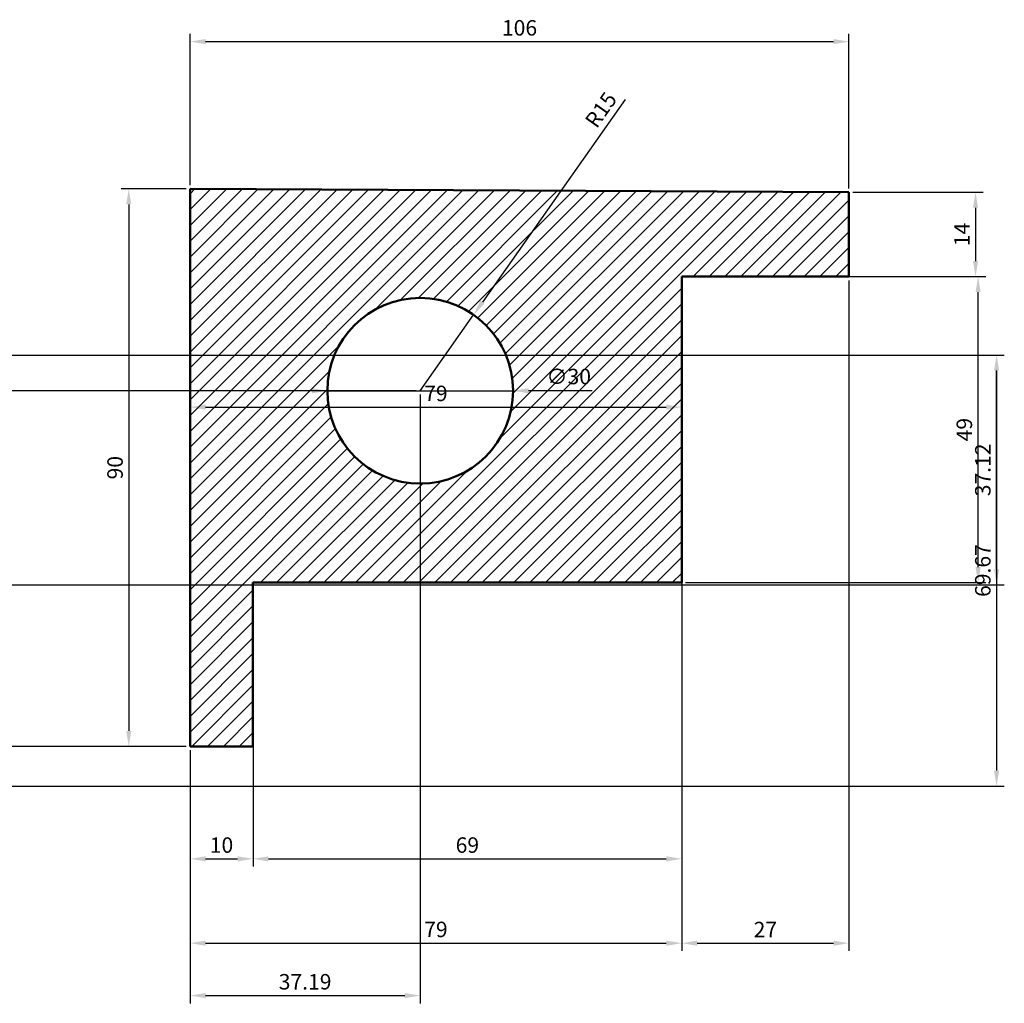
# Model space of a CAD drawing. Units: millimetres. Extents: x 1605 to 2079, y 1280 to 1879.
# Tile 6 of 7: x 1920 to 2079, y 1384 to 1543. Entities that reach past the tile are written whole.
import ezdxf

# ---------------------------------------------------------------- set-up
doc = ezdxf.new("R2010")
doc.units = ezdxf.units.MM
for name, color, linetype, lineweight in [('M-DIMS', 2, 'Continuous', 25), ('M-HATC', 8, 'Continuous', 18), ('M-OUTL', 7, 'Continuous', 50)]:
    doc.layers.add(name, color=color, linetype=linetype, lineweight=lineweight)
doc.styles.get("Standard").update_dxf_attribs({"font": 'arial.ttf'})
doc.dimstyles.new('ISO-25', dxfattribs={"dimtxt": 2.5, "dimasz": 2.5, "dimexe": 1.25, "dimexo": 0.625, "dimtad": 1, "dimdec": 0, "dimtxsty": 'Standard', "dimcen": 2.5, "dimadec": 0, "dimazin": 0, "dimtfac": 1, "dimtdec": 0, "dimtmove": 0, "dimatfit": 3, "dimfxl": 1, "dimarcsym": 0})

# ---------------------------------------------------------------- blocks, each defined once
blk = doc.blocks.new('*D30')
at = {"layer": 'Defpoints', "color": 0, "transparency": 16777216}
for p in [(1947.57, 1425.73), (1957.74, 1425.73), (1957.74, 1407.56)]:
    blk.add_point(p, dxfattribs=at)
at = {"layer": 'M-DIMS', "color": 0, "lineweight": -2, "transparency": 16777216}
for p, q in [((1947.57, 1425.11), (1947.57, 1406.31)), ((1957.74, 1425.11), (1957.74, 1406.31)), ((1950.07, 1407.56), (1955.24, 1407.56))]:
    blk.add_line(p, q, dxfattribs=at)
at = {"layer": 'M-DIMS', "color": 0, "transparency": 16777216}
for points in [[(1950.07, 1407.97), (1950.07, 1407.14), (1947.57, 1407.56)], [(1955.24, 1407.97), (1955.24, 1407.14), (1957.74, 1407.56)]]:
    blk.add_solid(points, dxfattribs=at)
at = {"layer": 'M-DIMS', "color": 0, "transparency": 16777216, "insert": (1952.65, 1409.46), "char_height": 2.5, "attachment_point": 5}
blk.add_mtext('10', dxfattribs=at)
blk = doc.blocks.new('*D31')
at = {"layer": 'Defpoints', "color": 0, "transparency": 16777216}
for p in [(1957.74, 1452.2), (2027.03, 1452.2), (2027.03, 1407.56)]:
    blk.add_point(p, dxfattribs=at)
at = {"layer": 'M-DIMS', "color": 0, "lineweight": -2, "transparency": 16777216}
for p, q in [((1957.74, 1451.57), (1957.74, 1406.31)), ((2027.03, 1451.57), (2027.03, 1406.31)), ((1960.24, 1407.56), (2024.53, 1407.56))]:
    blk.add_line(p, q, dxfattribs=at)
at = {"layer": 'M-DIMS', "color": 0, "transparency": 16777216}
for points in [[(1960.24, 1407.97), (1960.24, 1407.14), (1957.74, 1407.56)], [(2024.53, 1407.97), (2024.53, 1407.14), (2027.03, 1407.56)]]:
    blk.add_solid(points, dxfattribs=at)
at = {"layer": 'M-DIMS', "color": 0, "transparency": 16777216, "insert": (1992.38, 1409.46), "char_height": 2.5, "attachment_point": 5}
blk.add_mtext('69', dxfattribs=at)
blk = doc.blocks.new('*D32')
at = {"layer": 'Defpoints', "color": 0, "transparency": 16777216}
for p in [(2027.03, 1452.2), (1947.57, 1425.73), (2027.03, 1393.93)]:
    blk.add_point(p, dxfattribs=at)
at = {"layer": 'M-DIMS', "color": 0, "lineweight": -2, "transparency": 16777216}
for p, q in [((2027.03, 1451.57), (2027.03, 1392.68)), ((1947.57, 1425.11), (1947.57, 1392.68)), ((1950.07, 1393.93), (2024.53, 1393.93))]:
    blk.add_line(p, q, dxfattribs=at)
at = {"layer": 'M-DIMS', "color": 0, "transparency": 16777216}
for points in [[(1950.07, 1394.34), (1950.07, 1393.51), (1947.57, 1393.93)], [(2024.53, 1394.34), (2024.53, 1393.51), (2027.03, 1393.93)]]:
    blk.add_solid(points, dxfattribs=at)
at = {"layer": 'M-DIMS', "color": 0, "transparency": 16777216, "insert": (1987.3, 1395.83), "char_height": 2.5, "attachment_point": 5}
blk.add_mtext('79', dxfattribs=at)
blk = doc.blocks.new('*D33')
at = {"layer": 'Defpoints', "color": 0, "transparency": 16777216}
for p in [(2027.03, 1501.65), (2054.05, 1501.65), (2054.05, 1393.93)]:
    blk.add_point(p, dxfattribs=at)
at = {"layer": 'M-DIMS', "color": 0, "lineweight": -2, "transparency": 16777216}
for p, q in [((2027.03, 1501.02), (2027.03, 1392.68)), ((2054.05, 1501.02), (2054.05, 1392.68)), ((2029.53, 1393.93), (2051.55, 1393.93))]:
    blk.add_line(p, q, dxfattribs=at)
at = {"layer": 'M-DIMS', "color": 0, "transparency": 16777216}
for points in [[(2029.53, 1394.34), (2029.53, 1393.51), (2027.03, 1393.93)], [(2051.55, 1394.34), (2051.55, 1393.51), (2054.05, 1393.93)]]:
    blk.add_solid(points, dxfattribs=at)
at = {"layer": 'M-DIMS', "color": 0, "transparency": 16777216, "insert": (2040.54, 1395.81), "char_height": 2.5, "attachment_point": 5}
blk.add_mtext('27', dxfattribs=at)
blk = doc.blocks.new('*D34')
at = {"layer": 'Defpoints', "color": 0, "transparency": 16777216}
for p in [(2027.03, 1501.65), (2074.92, 1501.65), (2027.03, 1452.2)]:
    blk.add_point(p, dxfattribs=at)
at = {"layer": 'M-DIMS', "color": 0, "lineweight": -2, "transparency": 16777216}
for p, q in [((2027.65, 1501.65), (2076.17, 1501.65)), ((2074.92, 1454.7), (2074.92, 1499.15)), ((2027.65, 1452.2), (2076.17, 1452.2))]:
    blk.add_line(p, q, dxfattribs=at)
at = {"layer": 'M-DIMS', "color": 0, "transparency": 16777216}
for points in [[(2074.5, 1499.15), (2075.33, 1499.15), (2074.92, 1501.65)], [(2074.5, 1454.7), (2075.33, 1454.7), (2074.92, 1452.2)]]:
    blk.add_solid(points, dxfattribs=at)
at = {"layer": 'M-DIMS', "color": 0, "transparency": 16777216, "insert": (2073.01, 1476.92), "char_height": 2.5, "attachment_point": 5, "rotation": 90}
blk.add_mtext('49', dxfattribs=at)
blk = doc.blocks.new('*D35')
at = {"layer": 'Defpoints', "color": 0, "transparency": 16777216}
for p in [(2054.05, 1515.28), (2054.05, 1501.65), (2074.5, 1501.65)]:
    blk.add_point(p, dxfattribs=at)
at = {"layer": 'M-DIMS', "color": 0, "lineweight": -2, "transparency": 16777216}
for p, q in [((2054.67, 1515.28), (2075.75, 1515.28)), ((2074.5, 1512.78), (2074.5, 1504.15)), ((2054.67, 1501.65), (2075.75, 1501.65))]:
    blk.add_line(p, q, dxfattribs=at)
at = {"layer": 'M-DIMS', "color": 0, "transparency": 16777216}
for points in [[(2074.08, 1512.78), (2074.92, 1512.78), (2074.5, 1515.28)], [(2074.08, 1504.15), (2074.92, 1504.15), (2074.5, 1501.65)]]:
    blk.add_solid(points, dxfattribs=at)
at = {"layer": 'M-DIMS', "color": 0, "transparency": 16777216, "insert": (2072.62, 1508.46), "char_height": 2.5, "attachment_point": 5, "rotation": 90}
blk.add_mtext('14', dxfattribs=at)
blk = doc.blocks.new('*D36')
at = {"layer": 'Defpoints', "color": 0, "transparency": 16777216}
for p in [(2054.05, 1539.63), (1947.57, 1515.82), (2054.05, 1515.28)]:
    blk.add_point(p, dxfattribs=at)
at = {"layer": 'M-DIMS', "color": 0, "lineweight": -2, "transparency": 16777216}
for p, q in [((1947.57, 1516.44), (1947.57, 1540.88)), ((2054.05, 1515.91), (2054.05, 1540.88)), ((1950.07, 1539.63), (2051.55, 1539.63))]:
    blk.add_line(p, q, dxfattribs=at)
at = {"layer": 'M-DIMS', "color": 0, "transparency": 16777216}
for points in [[(1950.07, 1540.04), (1950.07, 1539.21), (1947.57, 1539.63)], [(2051.55, 1540.04), (2051.55, 1539.21), (2054.05, 1539.63)]]:
    blk.add_solid(points, dxfattribs=at)
at = {"layer": 'M-DIMS', "color": 0, "transparency": 16777216, "insert": (2000.81, 1541.53), "char_height": 2.5, "attachment_point": 5}
blk.add_mtext('106', dxfattribs=at)
blk = doc.blocks.new('*D37')
at = {"layer": 'Defpoints', "color": 0, "transparency": 16777216}
for p in [(1947.57, 1515.82), (1937.67, 1425.73), (1947.57, 1425.73)]:
    blk.add_point(p, dxfattribs=at)
at = {"layer": 'M-DIMS', "color": 0, "lineweight": -2, "transparency": 16777216}
for p, q in [((1946.94, 1515.82), (1936.42, 1515.82)), ((1937.67, 1513.32), (1937.67, 1428.23)), ((1946.94, 1425.73), (1936.42, 1425.73))]:
    blk.add_line(p, q, dxfattribs=at)
at = {"layer": 'M-DIMS', "color": 0, "transparency": 16777216}
for points in [[(1937.25, 1513.32), (1938.08, 1513.32), (1937.67, 1515.82)], [(1937.25, 1428.23), (1938.08, 1428.23), (1937.67, 1425.73)]]:
    blk.add_solid(points, dxfattribs=at)
at = {"layer": 'M-DIMS', "color": 0, "transparency": 16777216, "insert": (1935.77, 1470.77), "char_height": 2.5, "attachment_point": 5, "rotation": 90}
blk.add_mtext('90', dxfattribs=at)
blk = doc.blocks.new('*D38')
at = {"layer": 'Defpoints', "color": 0, "transparency": 16777216}
for p in [(2027.03, 1480.55), (2027.03, 1476.92), (1947.57, 1470.77)]:
    blk.add_point(p, dxfattribs=at)
at = {"layer": 'M-DIMS', "color": 0, "lineweight": -2, "transparency": 16777216}
for p, q in [((1947.57, 1471.4), (1947.57, 1481.8)), ((2027.03, 1477.55), (2027.03, 1481.8)), ((1950.07, 1480.55), (2024.53, 1480.55))]:
    blk.add_line(p, q, dxfattribs=at)
at = {"layer": 'M-DIMS', "color": 0, "transparency": 16777216}
for points in [[(1950.07, 1480.97), (1950.07, 1480.14), (1947.57, 1480.55)], [(2024.53, 1480.97), (2024.53, 1480.14), (2027.03, 1480.55)]]:
    blk.add_solid(points, dxfattribs=at)
at = {"layer": 'M-DIMS', "color": 0, "transparency": 16777216, "insert": (1987.3, 1482.45), "char_height": 2.5, "attachment_point": 5}
blk.add_mtext('79', dxfattribs=at)
blk = doc.blocks.new('*D39')
at = {"layer": 'Defpoints', "color": 0, "transparency": 16777216}
for p in [(1993.39, 1495.47), (1984.76, 1483.2)]:
    blk.add_point(p, dxfattribs=at)
at = {"layer": 'M-DIMS', "color": 0, "lineweight": -2, "transparency": 16777216}
for p, q in [((2017.87, 1530.29), (1994.82, 1497.52)), ((1984.76, 1483.2), (1993.39, 1495.47))]:
    blk.add_line(p, q, dxfattribs=at)
at = {"layer": 'M-DIMS', "color": 0, "transparency": 16777216}
blk.add_solid([(1994.48, 1497.76), (1995.16, 1497.28), (1993.39, 1495.47)], dxfattribs=at)
at = {"layer": 'M-DIMS', "color": 0, "transparency": 16777216, "insert": (2014.23, 1528.42), "char_height": 2.5, "attachment_point": 5, "rotation": 54.8827}
blk.add_mtext('R15', dxfattribs=at)
blk = doc.blocks.new('*D40')
at = {"layer": 'Defpoints', "color": 0, "transparency": 16777216}
for p in [(1916.42, 1488.98), (1783.42, 1419.31), (2077.9, 1419.31)]:
    blk.add_point(p, dxfattribs=at)
at = {"layer": 'M-DIMS', "color": 0, "lineweight": -2, "transparency": 16777216}
for p, q in [((1917.04, 1488.98), (2079.15, 1488.98)), ((2077.9, 1486.48), (2077.9, 1421.81)), ((1784.04, 1419.31), (2079.15, 1419.31))]:
    blk.add_line(p, q, dxfattribs=at)
at = {"layer": 'M-DIMS', "color": 0, "transparency": 16777216}
for points in [[(2077.48, 1486.48), (2078.32, 1486.48), (2077.9, 1488.98)], [(2077.48, 1421.81), (2078.32, 1421.81), (2077.9, 1419.31)]]:
    blk.add_solid(points, dxfattribs=at)
at = {"layer": 'M-DIMS', "color": 0, "transparency": 16777216, "insert": (2076, 1454.15), "char_height": 2.5, "attachment_point": 5, "rotation": 90}
blk.add_mtext('69.67', dxfattribs=at)
blk = doc.blocks.new('*D46')
at = {"layer": 'Defpoints', "color": 0, "transparency": 16777216}
for p in [(1883.42, 1488.98), (2077.9, 1488.98), (1837.61, 1451.86)]:
    blk.add_point(p, dxfattribs=at)
at = {"layer": 'M-DIMS', "color": 0, "lineweight": -2, "transparency": 16777216}
for p, q in [((1884.04, 1488.98), (2079.15, 1488.98)), ((2077.9, 1454.36), (2077.9, 1486.48)), ((1838.23, 1451.86), (2079.15, 1451.86))]:
    blk.add_line(p, q, dxfattribs=at)
at = {"layer": 'M-DIMS', "color": 0, "transparency": 16777216}
for points in [[(2077.48, 1486.48), (2078.32, 1486.48), (2077.9, 1488.98)], [(2077.48, 1454.36), (2078.32, 1454.36), (2077.9, 1451.86)]]:
    blk.add_solid(points, dxfattribs=at)
at = {"layer": 'M-DIMS', "color": 0, "transparency": 16777216, "insert": (2076, 1470.42), "char_height": 2.5, "attachment_point": 5, "rotation": 90}
blk.add_mtext('37.12', dxfattribs=at)
blk = doc.blocks.new('*D50')
at = {"layer": 'Defpoints', "color": 0, "transparency": 16777216}
for p in [(1984.76, 1483.2), (1947.57, 1425.73), (1984.76, 1385.46)]:
    blk.add_point(p, dxfattribs=at)
at = {"layer": 'M-DIMS', "color": 0, "lineweight": -2, "transparency": 16777216}
for p, q in [((1984.76, 1482.58), (1984.76, 1384.21)), ((1947.57, 1425.11), (1947.57, 1384.21)), ((1950.07, 1385.46), (1982.26, 1385.46))]:
    blk.add_line(p, q, dxfattribs=at)
at = {"layer": 'M-DIMS', "color": 0, "transparency": 16777216}
for points in [[(1950.07, 1385.88), (1950.07, 1385.05), (1947.57, 1385.46)], [(1982.26, 1385.88), (1982.26, 1385.05), (1984.76, 1385.46)]]:
    blk.add_solid(points, dxfattribs=at)
at = {"layer": 'M-DIMS', "color": 0, "transparency": 16777216, "insert": (1966.16, 1387.37), "char_height": 2.5, "attachment_point": 5}
blk.add_mtext('37.19', dxfattribs=at)
blk = doc.blocks.new('*D51')
at = {"layer": 'Defpoints', "color": 0, "transparency": 16777216}
for p in [(1624.07, 1483.2), (1984.76, 1483.2), (1947.57, 1425.73)]:
    blk.add_point(p, dxfattribs=at)
at = {"layer": 'M-DIMS', "color": 0, "lineweight": -2, "transparency": 16777216}
for p, q in [((1984.13, 1483.2), (1622.82, 1483.2)), ((1624.07, 1428.23), (1624.07, 1480.7)), ((1946.94, 1425.73), (1622.82, 1425.73))]:
    blk.add_line(p, q, dxfattribs=at)
at = {"layer": 'M-DIMS', "color": 0, "transparency": 16777216}
for points in [[(1623.65, 1480.7), (1624.48, 1480.7), (1624.07, 1483.2)], [(1623.65, 1428.23), (1624.48, 1428.23), (1624.07, 1425.73)]]:
    blk.add_solid(points, dxfattribs=at)
at = {"layer": 'M-DIMS', "color": 0, "transparency": 16777216, "insert": (1622.17, 1454.47), "char_height": 2.5, "attachment_point": 5, "rotation": 90}
blk.add_mtext('57.47', dxfattribs=at)
blk = doc.blocks.new('*D70')
at = {"layer": 'Defpoints', "color": 0, "transparency": 16777216}
for p in [(1969.76, 1483.2), (1999.76, 1483.2)]:
    blk.add_point(p, dxfattribs=at)
at = {"layer": 'M-DIMS', "color": 0, "lineweight": -2, "transparency": 16777216}
for p, q in [((1967.26, 1483.2), (1964.76, 1483.2)), ((1969.76, 1483.2), (1999.76, 1483.2)), ((2012.53, 1483.21), (2002.26, 1483.2))]:
    blk.add_line(p, q, dxfattribs=at)
at = {"layer": 'M-DIMS', "color": 0, "transparency": 16777216}
for points in [[(1967.26, 1483.62), (1967.26, 1482.79), (1969.76, 1483.2)], [(2002.26, 1483.62), (2002.26, 1482.79), (1999.76, 1483.2)]]:
    blk.add_solid(points, dxfattribs=at)
at = {"layer": 'M-DIMS', "color": 0, "transparency": 16777216, "insert": (2008.76, 1485.18), "char_height": 2.5, "attachment_point": 5, "rotation": 0.0016}
blk.add_mtext('∅30', dxfattribs=at)

msp = doc.modelspace()

# ---------------------------------------------------------------- hatches: boundary and pattern name
at = {"layer": 'M-HATC'}
h = msp.add_hatch(dxfattribs=at)
h.set_pattern_fill('ANSI31', color=256, scale=0.57)
h.paths.add_polyline_path([(2027.0272, 1501.6485), (2054.0484, 1501.6485), (2054.0484, 1515.281), (1947.5688, 1515.8156), (1947.5688, 1425.7344), (1957.7352, 1425.7344), (1957.7352, 1452.1974), (2027.0272, 1452.1974)])
h.paths.add_polyline_path([(1999.7564, 1483.2046, -1), (1969.7564, 1483.2046, -1)], flags=16)

# ---------------------------------------------------------------- linework, layer by layer
at = {"layer": 'M-OUTL'}
for p, q in [((1947.5688, 1515.8156), (1947.5688, 1425.7344)), ((2054.0484, 1515.281), (1947.5688, 1515.8156)), ((2054.0484, 1501.6485), (2054.0484, 1515.281)), ((2027.0272, 1452.1974), (2027.0272, 1501.6485)), ((2027.0272, 1501.6485), (2054.0484, 1501.6485)), ((1957.7352, 1425.7344), (1957.7352, 1452.1974)), ((1957.7352, 1452.1974), (2027.0272, 1452.1974)), ((1947.5688, 1425.7344), (1957.7352, 1425.7344))]:
    msp.add_line(p, q, dxfattribs=at)
msp.add_circle((1984.7564, 1483.2046), 15, dxfattribs=at)

# ---------------------------------------------------------------- dimensions: what is measured, and where the dimension line sits
at = {"layer": 'M-DIMS'}
for base, p1, p2, override, picture, middle in [((2054.0484, 1539.6258), (1947.5688, 1515.8156), (2054.0484, 1515.281), {"dimclrd": 0, "dimclre": 0, "dimclrt": 0}, '*D36', (2000.8086, 1541.5272)), ((2054.0484, 1393.9253), (2027.0272, 1501.6485), (2054.0484, 1501.6485), {"dimclrd": 0, "dimclre": 0, "dimclrt": 0}, '*D33', (2040.5378, 1395.8054)), ((2027.0272, 1480.5518), (1947.5688, 1470.775), (2027.0272, 1476.923), {"dimclrd": 0, "dimclre": 0, "dimclrt": 0}, '*D38', (1987.298, 1482.4532)), ((1984.7564, 1385.4644), (1947.5688, 1425.7344), (1984.7564, 1483.2046), {"dimdec": 2, "dimlfac": 1, "dimrnd": 0, "dimzin": 0, "dimdsep": 46, "dimlunit": 2}, '*D50', (1966.1626, 1387.3667)), ((2027.0272, 1393.9253), (1947.5688, 1425.7344), (2027.0272, 1452.1974), {"dimclrd": 0, "dimclre": 0, "dimclrt": 0}, '*D32', (1987.298, 1395.8268)), ((2027.0272, 1407.5578), (1957.7352, 1452.1974), (2027.0272, 1452.1974), {"dimclrd": 0, "dimclre": 0, "dimclrt": 0}, '*D31', (1992.3812, 1409.4592)), ((1957.7352, 1407.5578), (1947.5688, 1425.7344), (1957.7352, 1425.7344), {"dimclrd": 0, "dimclre": 0, "dimclrt": 0}, '*D30', (1952.652, 1409.4592))]:
    dim = msp.add_linear_dim(base=base, p1=p1, p2=p2, dimstyle='ISO-25', override=override, dxfattribs=at)
    dim.commit()
    dim.dimension.update_dxf_attribs({"geometry": picture, "text_midpoint": middle})
dim = msp.add_radius_dim(center=(1984.7564, 1483.2046), mpoint=(1993.3851, 1495.4742), dimstyle='ISO-25', override={"dimclrd": 0, "dimclre": 0, "dimclrt": 0}, dxfattribs=at)
dim.commit()
dim.dimension.update_dxf_attribs({"geometry": '*D39', "text_midpoint": (2015.788, 1527.3298), "dimtype": 164})
for base, p1, p2, override, picture, middle in [((1937.6672, 1425.7344), (1947.5688, 1515.8156), (1947.5688, 1425.7344), {"dimclrd": 0, "dimclre": 0, "dimclrt": 0}, '*D37', (1935.7658, 1470.775)), ((2074.4996, 1501.6485), (2054.0484, 1515.281), (2054.0484, 1501.6485), {"dimclrd": 0, "dimclre": 0, "dimclrt": 0}, '*D35', (2072.6195, 1508.4647)), ((2074.9163, 1501.6485), (2027.0272, 1452.1974), (2027.0272, 1501.6485), {"dimclrd": 0, "dimclre": 0, "dimclrt": 0}, '*D34', (2073.0148, 1476.923)), ((2077.8984, 1419.3145), (1916.4159, 1488.9806), (1783.4159, 1419.3145), {"dimdec": 2, "dimlfac": 1, "dimrnd": 0, "dimzin": 0, "dimdsep": 46, "dimlunit": 2}, '*D40', (2075.997, 1454.1475)), ((2077.8984, 1488.9806), (1837.6066, 1451.8622), (1883.4159, 1488.9806), {"dimdec": 2, "dimlfac": 1, "dimrnd": 0, "dimzin": 0, "dimdsep": 46, "dimlunit": 2}, '*D46', (2075.9961, 1470.4214)), ((1624.0659, 1483.2046), (1947.5688, 1425.7344), (1984.7564, 1483.2046), {"dimdec": 2, "dimlfac": 1, "dimrnd": 0, "dimzin": 0, "dimdsep": 46, "dimlunit": 2}, '*D51', (1622.1695, 1454.4695))]:
    dim = msp.add_linear_dim(base=base, p1=p1, p2=p2, angle=90, dimstyle='ISO-25', override=override, dxfattribs=at)
    dim.commit()
    dim.dimension.update_dxf_attribs({"geometry": picture, "text_midpoint": middle})
dim = msp.add_diameter_dim_2p(p1=(1969.7564, 1483.2042), p2=(1999.7564, 1483.205), dimstyle='ISO-25', override={"dimdec": 0, "dimlfac": 1, "dimrnd": 0, "dimzin": 0, "dimdsep": 46, "dimlunit": 2}, dxfattribs=at)
dim.commit()
dim.dimension.update_dxf_attribs({"geometry": '*D70', "text_midpoint": (2008.7564, 1483.2053), "dimtype": 163})

doc.saveas('drawing.dxf')
